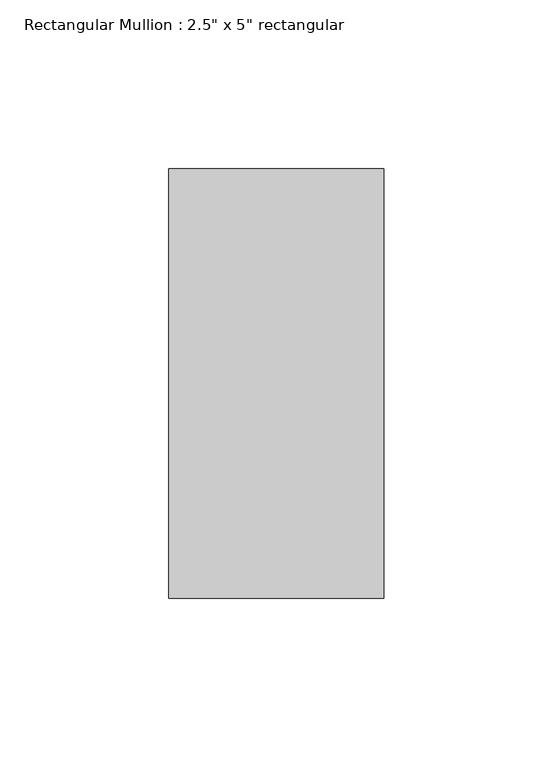
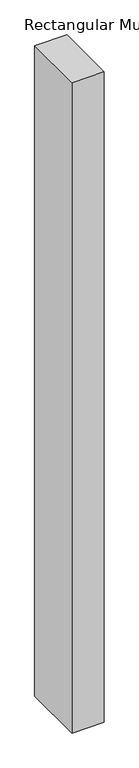
"""IFC4 building model written with IfcOpenShell, lengths in millimetres: member geometry."""

from ifc_helpers import new_model, si_unit, frame, origin, place, context, project, spatial, polyline, outline, extrude, source, transform, mapped, element, save


def member_20eb5ac3(model_context):
    return source(origin(), model_context, "Body", "SweptSolid", [
        extrude(outline(polyline([(0.0, 63.5), (0.0, -63.5), (-63.5, -63.5), (-63.5, 63.5), (0.0, 63.5)])), frame((0.0, 0.0, -1352.55), z_axis=(0.0, 0.0, 1.0), x_axis=(1.0, 0.0, 0.0)), (0.0, 0.0, 1.0), 1352.55),
    ])


if __name__ == "__main__":
    model = new_model("IFC4")
    model_context = context("Model", 3, world=origin())
    ifc_project = project(units=[si_unit("LENGTHUNIT", "METRE", prefix="MILLI")], contexts=[model_context])
    site = spatial("IfcSite", under=ifc_project)
    building = spatial("IfcBuilding", under=site)
    placement = place(None, origin())
    member_shape = member_20eb5ac3(model_context)
    element("IfcMember", 1, ObjectType="Rectangular Mullion : 2.5\" x 5\" rectangular", at=placement, inside=building, context=model_context, shape_type="MappedRepresentation", body=[
        mapped(member_shape, transform((0.0, 0.0, 0.0), x_axis=(1.0, 0.0, 0.0), y_axis=(0.0, 1.0, 0.0), z_axis=(0.0, 0.0, 1.0))),
    ])
    save(model, "model.ifc")

# Revit data of these elements
# Type "Rectangular Mullion : 2.5\" x 5\" rectangular"
#   built-in parameter 1007304 = 0.416667 (stored number, unit not read)
#   built-in parameter 1007301 = 0.104167 (stored number, unit not read)
#   built-in parameter 1007300 = 0.104167 (stored number, unit not read)
# Element 1 (IfcMember, "Rectangular Mullion : 2.5\" x 5\" rectangular")
#   Materials on its faces: "Aluminum"
# Materials
#   "Aluminum": class "Metal", colour RGB 247 247 247, transparency 0, Description = "Aluminum 6061", Cost = 0
